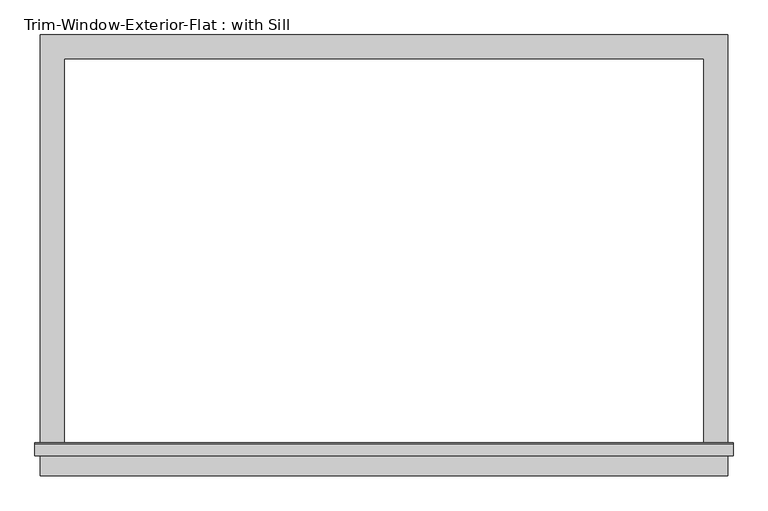
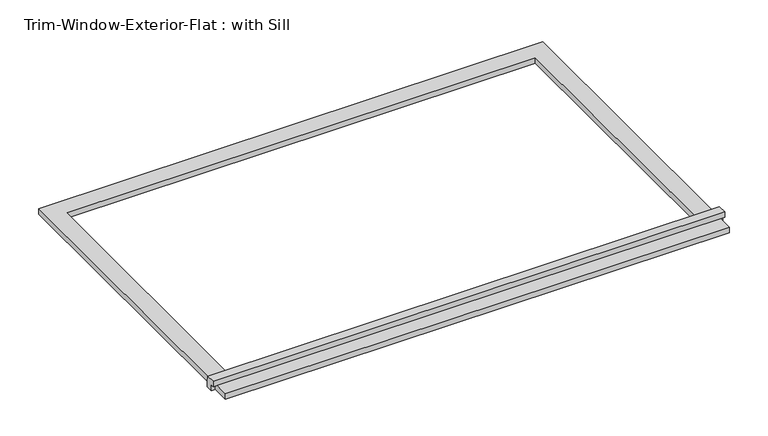
"""IFC4 building model written with IfcOpenShell, lengths in millimetres: proxy geometry, Trim-Window-Exterior-Flat : with Sill."""

from ifc_helpers import new_model, si_unit, frame, origin, origin_with_axes, place, context, project, spatial, polyline, outline, extrude, source, transform, mapped, element, save


def trim_window_exterior_flat_with_sill_979bde60(model_context):
    return source(origin(), model_context, "Body", "SweptSolid", [
        extrude(outline(polyline([(819.15, -936.5823709), (819.15, -993.7323709), (-819.15, -993.7323709), (-819.15, -936.5823709), (819.15, -936.5823709)])), origin_with_axes(), (0.0, 0.0, 1.0), 19.05),
        extrude(outline(polyline([(-946.15, 38.1), (-916.8580645, 38.1), (-914.4, 19.05), (-914.4, 0.0), (-936.5823709, 0.0), (-936.5823709, 19.05), (-946.15, 19.05), (-946.15, 38.1)])), frame((-831.85, 0.0, 0.0), z_axis=(1.0, 0.0, 0.0), x_axis=(0.0, 1.0, 0.0)), (0.0, 0.0, 1.0), 1663.7),
        extrude(outline(polyline([(-819.15, 57.15), (819.15, 57.15), (819.15, -914.4), (762.0, -914.4), (762.0, 0.0), (-762.0, 0.0), (-762.0, -914.4), (-819.15, -914.4), (-819.15, 57.15)])), origin_with_axes(), (0.0, 0.0, 1.0), 19.05),
    ])


if __name__ == "__main__":
    model = new_model("IFC4")
    model_context = context("Model", 3, world=origin())
    ifc_project = project(units=[si_unit("LENGTHUNIT", "METRE", prefix="MILLI")], contexts=[model_context])
    site = spatial("IfcSite", under=ifc_project)
    building = spatial("IfcBuilding", under=site)
    placement = place(None, origin())
    trim_window_exterior_flat_with_sill_shape = trim_window_exterior_flat_with_sill_979bde60(model_context)
    element("IfcBuildingElementProxy", 1, Name="Trim-Window-Exterior-Flat : with Sill", ObjectType="Trim-Window-Exterior-Flat : with Sill", at=placement, inside=building, context=model_context, shape_type="MappedRepresentation", body=[
        mapped(trim_window_exterior_flat_with_sill_shape, transform((0.0, 0.0, 0.0), x_axis=(1.0, 0.0, 0.0), y_axis=(0.0, 1.0, 0.0), z_axis=(0.0, 0.0, 1.0))),
    ])
    save(model, "model.ifc")

# Revit data of these elements
# Type "Trim-Window-Exterior-Flat : with Sill"
#   Trim Width = 0' - 2 1/4"
#   Trim Thickness_Picture Frame = 0' - 1 1/4"
#   Trim Thickness_with Sill = 0' - 0 3/4"
#   Sill Thickness = 0' - 1 1/4"
#   Opening Width [instance default] = 2' - 0"
#   Opening Height [instance default] = 3' - 0"
#   Default Elevation = 4' - 0"
#   Sill = yes
#   Picture Frame = no
#   Trim Material [instance default] = none
# Element 1 (IfcBuildingElementProxy, "Trim-Window-Exterior-Flat : with Sill")
#   Opening Width = 5' - 0"
#   Trim Material = Clad - White
#   Materials on its faces: "Clad - White"
# Materials
#   "Clad - White": class "Wood", colour RGB 242 242 238, transparency 0, Cost = 0
